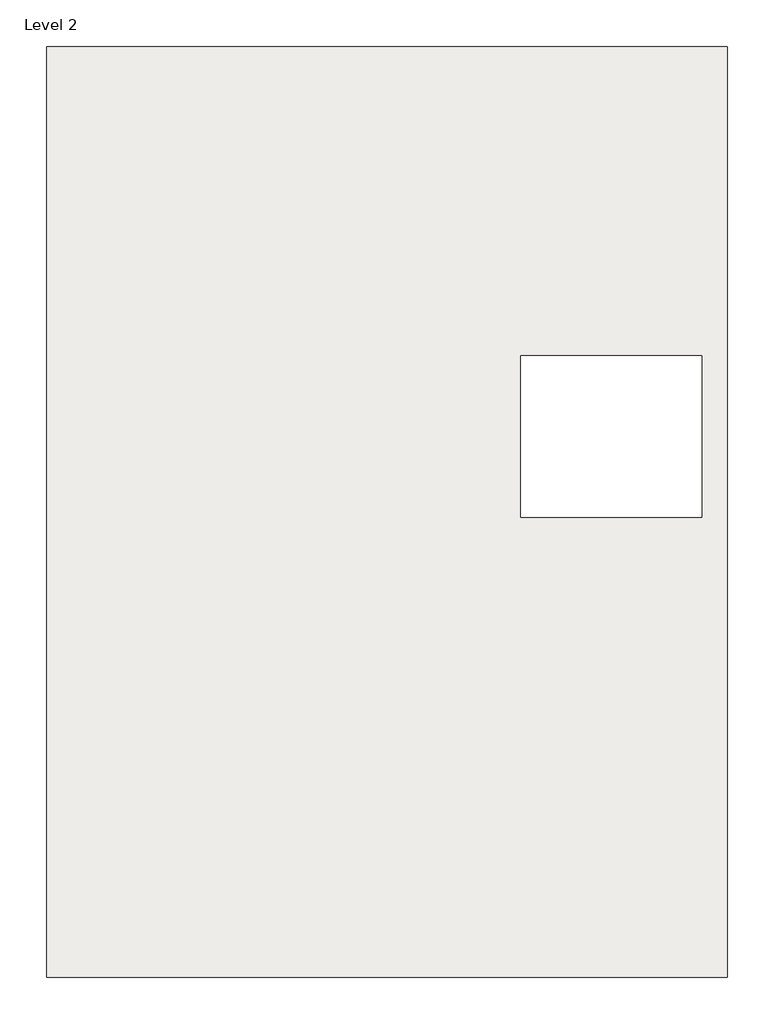
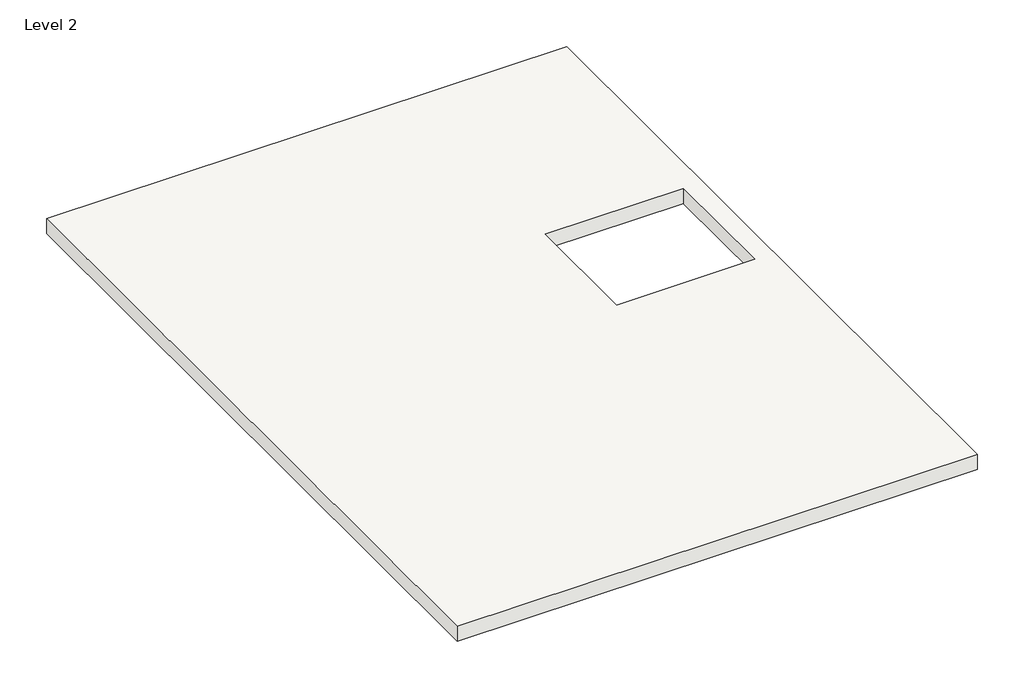
# One storey: 1 roof.
"""IFC4 building model written with IfcOpenShell, lengths in millimetres."""

from ifc_helpers import new_model, si_unit, frame, origin, place, context, project, spatial, polyline, outline, extrude, element, save

model = new_model("IFC4")

# Units and contexts
model_context = context("Model", 3, world=origin())
ifc_project = project(units=[si_unit("LENGTHUNIT", "METRE", prefix="MILLI")], contexts=[model_context])

# Site, building, storey
site = spatial("IfcSite", under=ifc_project)
building = spatial("IfcBuilding", under=site)
storey = spatial("IfcBuildingStorey", under=building, Name="Level 2", Elevation=3048.0)

# Roof
placement = place(None, origin())
element("IfcRoof", 1, ObjectType="Generic - 12\"", at=placement, inside=storey, context=model_context, shape_type="SweptSolid", body=[
    extrude(outline(polyline([(-14810.1837964, 11764.1759458), (-4853.3837964, 11764.1759458), (-4853.3837964, -1850.2240542), (-14810.1837964, -1850.2240542), (-14810.1837964, 11764.1759458)]), holes=[polyline([(-5230.9965416, 7240.6036881), (-7872.5965416, 7240.6036881), (-7872.5965416, 4878.4036881), (-5230.9965416, 4878.4036881), (-5230.9965416, 7240.6036881)])]), frame((0.0, 0.0, 3048.0), z_axis=(0.0, 0.0, 1.0), x_axis=(1.0, 0.0, 0.0)), (0.0, 0.0, 1.0), 304.8),
])

save(model, "model.ifc")

# Revit data of these elements
# Type "Generic - 12\""
#   Assembly Code = "B1020"
#   Layers, outside or top first: 1' - 0" "Brick, Soldier Course" (function 1)
# Element 1 (IfcRoof, "Generic - 12\"")
#   built-in parameter 1001705 = 11 (stored number, unit not read)
#   built-in parameter 1001710 = 33615
#   Phase Created = New Construction
#   Materials on its faces: "Brick, Soldier Course"
# Materials
#   "Brick, Soldier Course": class "Masonry", colour RGB 170 98 104, transparency 0, Description = "Common brick soldier coursed", Cost = 0
